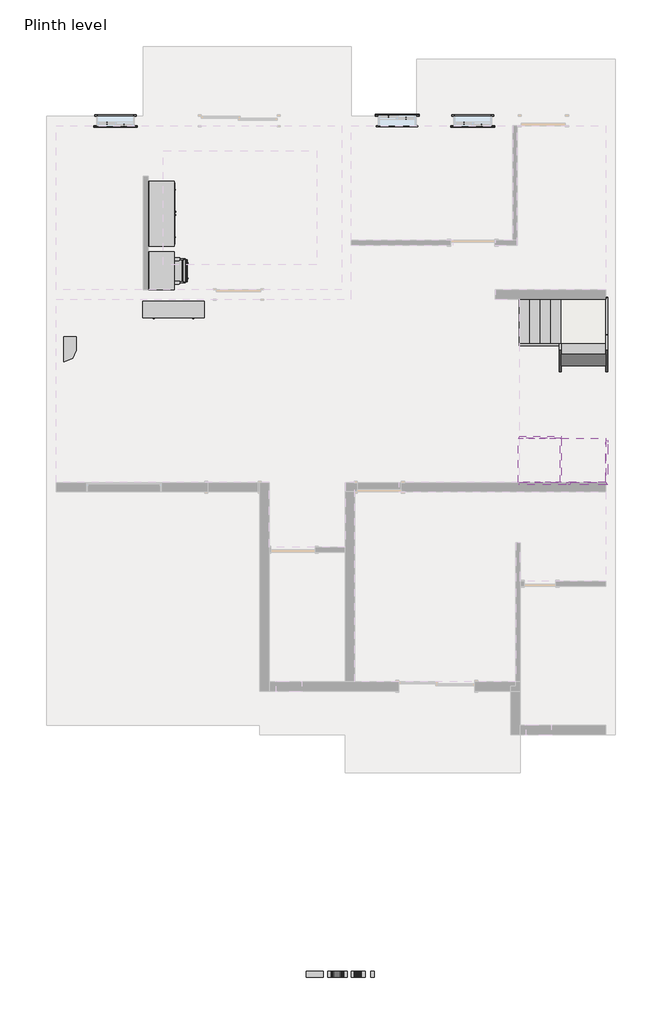
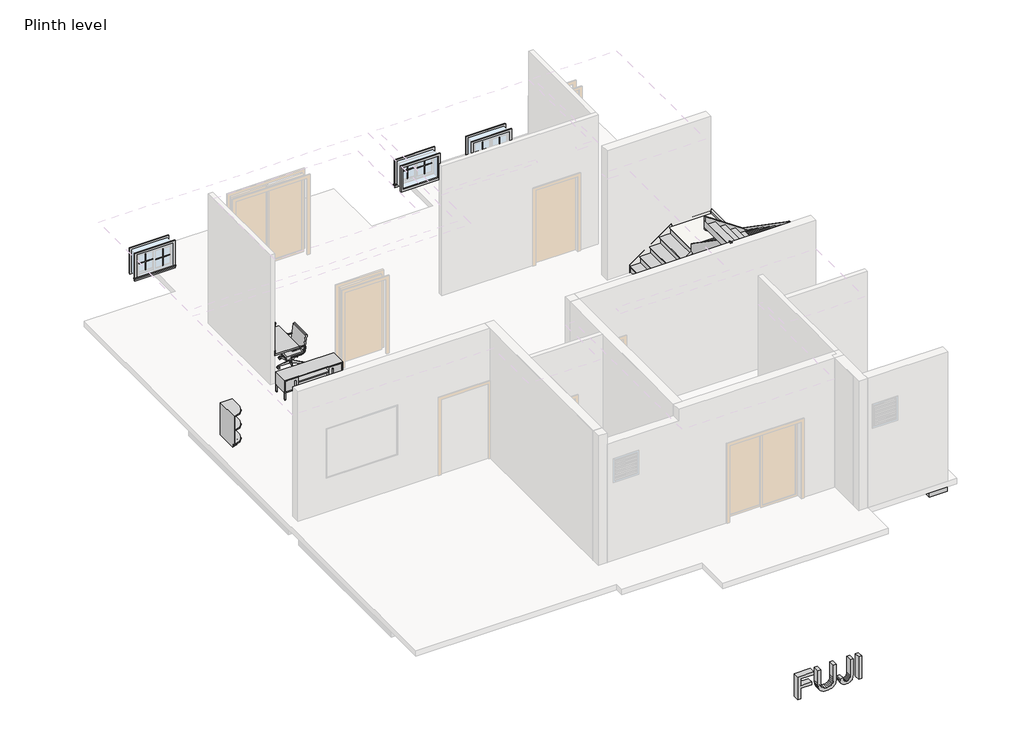
# One storey, part 2 of 2: 25 proxies, 10 members, 7 beams, 6 furniture elements, 3 stair flights, 2 slabs.
"""IFC4 building model written with IfcOpenShell, lengths in millimetres."""

from ifc_helpers import new_model, si_unit, frame, origin, place, context, project, spatial, polyline, outline, extrude, faceted_brep, transform, mapped, element, save
from components import muntin_pattern_2x2_muntin_pattern_2x2_87da473c, trim_window_exterior_flat_with_sill_40e754a6, trim_window_interior_flat_picture_frame_6592d821, furniture_d2b2b685, furniture_4ce329b2, chair_task_arms_chair_task_arms_bb362225, tv_stand_17254_tv_stand_17254_2bb553a4, furniture_0c89dcb9, furniture_49332987, non_monolithic_landing_caa31a54, non_monolithic_landing_665b62c1, stair_flight_49469ed7, stair_flight_6a237a90, stair_flight_f733f96e

model = new_model("IFC4")

# Units and contexts
model_context = context("Model", 3, world=origin())
ifc_project = project(units=[si_unit("LENGTHUNIT", "METRE", prefix="MILLI")], contexts=[model_context])

# Site, building, storey
site = spatial("IfcSite", under=ifc_project)
building = spatial("IfcBuilding", under=site)
storey = spatial("IfcBuildingStorey", under=building, Name="Plinth level", Elevation=0.0)

# Beams
placement = place(None, origin())
element("IfcBeam", 1, ObjectType="Concrete-Rectangular Beam : 18X12", at=placement, inside=storey, context=model_context, shape_type="Brep", body=[
    faceted_brep([(5601.0916032, 10641.5241878, -152.4), (5601.0916032, 10184.3241878, -152.4), (12153.8099466, 10184.3241878, -152.4), (12611.0099466, 10184.3241878, -152.4), (12611.0099466, 10412.9241878, -152.4), (12382.4099466, 10412.9241878, -152.4), (12382.4099466, 10641.5241878, -152.4), (7823.1099466, 10641.5241878, -152.4), (7823.1099466, 10412.9241878, -152.4), (7594.5099466, 10412.9241878, -152.4), (7594.5099466, 10641.5241878, -152.4), (5601.0916032, 10184.3241878, -457.2), (12153.8099466, 10184.3241878, -457.2), (12611.0099466, 10184.3241878, -457.2), (5601.0916032, 10641.5241878, -457.2), (7594.5099466, 10641.5241878, -457.2), (7594.5099466, 10412.9241878, -457.2), (7823.1099466, 10412.9241878, -457.2), (7823.1099466, 10641.5241878, -457.2), (12382.4099466, 10641.5241878, -457.2), (12382.4099466, 10412.9241878, -457.2), (12611.0099466, 10412.9241878, -457.2)], [[[0, 1, 2, 3, 4, 5, 6, 7, 8, 9, 10]], [[1, 11, 12, 13, 3, 2]], [[11, 14, 15, 16, 17, 18, 19, 20, 21, 13, 12]], [[6, 19, 18, 7]], [[0, 14, 11, 1]], [[3, 13, 21, 4]], [[20, 5, 4, 21]], [[5, 20, 19, 6]], [[17, 8, 7, 18]], [[8, 17, 16, 9]], [[9, 16, 15, 10]], [[14, 0, 10, 15]]]),
])
element("IfcBeam", 2, ObjectType="Concrete-Rectangular Beam : 18X12", at=placement, inside=storey, context=model_context, shape_type="Brep", body=[
    faceted_brep([(12611.0099466, 10184.3241878, -152.4), (18402.6916032, 10184.3241878, -152.4), (18859.8916032, 10184.3241878, -152.4), (18859.8916032, 10412.9241878, -152.4), (18402.6916032, 10412.9241878, -152.4), (18402.6916032, 10641.5241878, -152.4), (12839.6099466, 10641.5241878, -152.4), (12839.6099466, 10412.9241878, -152.4), (12611.0099466, 10412.9241878, -152.4), (18859.8916032, 10184.3241878, -457.2), (12611.0099466, 10184.3241878, -457.2), (18402.6916032, 10184.3241878, -457.2), (12611.0099466, 10412.9241878, -457.2), (12839.6099466, 10412.9241878, -457.2), (12839.6099466, 10641.5241878, -457.2), (18402.6916032, 10641.5241878, -457.2), (18402.6916032, 10412.9241878, -457.2), (18859.8916032, 10412.9241878, -457.2)], [[[0, 1, 2, 3, 4, 5, 6, 7, 8]], [[9, 2, 1, 0, 10, 11]], [[9, 11, 10, 12, 13, 14, 15, 16, 17]], [[14, 6, 5, 15]], [[2, 9, 17, 3]], [[10, 0, 8, 12]], [[13, 7, 6, 14]], [[7, 13, 12, 8]], [[16, 4, 3, 17]], [[4, 16, 15, 5]]]),
])
element("IfcBeam", 3, ObjectType="Concrete-Rectangular Beam : 18X12", at=placement, inside=storey, context=model_context, shape_type="Brep", body=[
    faceted_brep([(18859.8916032, 10184.3241878, -152.4), (18402.6916032, 10184.3241878, -152.4), (18402.6916032, 6450.5241878, -152.4), (18823.689508, 6450.5241878, -152.4), (18823.689508, 6221.9241878, -152.4), (18402.6916032, 6221.9241878, -152.4), (18402.6916032, 1802.3241878, -152.4), (18859.8916032, 1802.3241878, -152.4), (18402.6916032, 10184.3241878, -457.2), (18402.6916032, 6450.5241878, -457.2), (18859.8916032, 10184.3241878, -457.2), (18859.8916032, 1802.3241878, -457.2), (18402.6916032, 1802.3241878, -457.2), (18402.6916032, 6221.9241878, -457.2), (18823.689508, 6221.9241878, -457.2), (18823.689508, 6450.5241878, -457.2)], [[[0, 1, 2, 3, 4, 5, 6, 7]], [[1, 8, 9, 2]], [[8, 10, 11, 12, 13, 14, 15, 9]], [[10, 0, 7, 11]], [[1, 0, 10, 8]], [[15, 3, 2, 9]], [[3, 15, 14, 4]], [[4, 14, 13, 5]], [[7, 6, 12, 11]], [[5, 13, 12, 6]]]),
    faceted_brep([(18859.8916032, -4052.3758122, -152.4), (18402.6916032, -4052.3758122, -152.4), (18402.6916032, -4052.3758122, -457.2), (18859.8916032, -4052.3758122, -457.2), (18402.6916032, -3226.8758122, -152.4), (18402.6916032, -2769.6758122, -152.4), (18402.6916032, 1345.1241878, -152.4), (18402.6916032, 1573.7241878, -152.4), (18402.6916032, 1573.7241878, -457.2), (18402.6916032, 1345.1241878, -457.2), (18402.6916032, -2769.6758122, -457.2), (18402.6916032, -3226.8758122, -457.2), (18859.8916032, 1573.7241878, -152.4), (18859.8916032, 1573.7241878, -457.2)], [[[0, 1, 2, 3]], [[2, 1, 4, 5, 6, 7, 8, 9, 10, 11]], [[7, 12, 13, 8]], [[1, 0, 12, 7, 6, 5, 4]], [[3, 2, 11, 10, 9, 8, 13]], [[0, 3, 13, 12]]]),
])
element("IfcBeam", 4, ObjectType="Concrete-Rectangular Beam : 18X12", at=placement, inside=storey, context=model_context, shape_type="Brep", body=[
    faceted_brep([(12611.0099466, 6679.1241878, -152.4), (12153.8099466, 6679.1241878, -152.4), (5829.6916032, 6679.1241878, -152.4), (5829.6916032, 6221.9241878, -152.4), (7480.2099466, 6221.9241878, -152.4), (7480.2099466, 6450.5241878, -152.4), (7708.8099466, 6450.5241878, -152.4), (7708.8099466, 6221.9241878, -152.4), (12153.8099466, 6221.9241878, -152.4), (12153.8099466, 6450.5241878, -152.4), (12611.0099466, 6450.5241878, -152.4), (12153.8099466, 6221.9241878, -457.2), (7708.8099466, 6221.9241878, -457.2), (5829.6916032, 6679.1241878, -457.2), (12153.8099466, 6679.1241878, -457.2), (12611.0099466, 6679.1241878, -457.2), (12611.0099466, 6450.5241878, -457.2), (12153.8099466, 6450.5241878, -457.2), (7708.8099466, 6450.5241878, -457.2), (7480.2099466, 6450.5241878, -457.2), (7480.2099466, 6221.9241878, -457.2), (5829.6916032, 6221.9241878, -457.2)], [[[0, 1, 2, 3, 4, 5, 6, 7, 8, 9, 10]], [[11, 8, 7, 12]], [[13, 14, 15, 16, 17, 11, 12, 18, 19, 20, 21]], [[0, 15, 14, 13, 2, 1]], [[3, 2, 13, 21]], [[15, 0, 10, 16]], [[9, 17, 16, 10]], [[17, 9, 8, 11]], [[6, 18, 12, 7]], [[19, 5, 4, 20]], [[5, 19, 18, 6]], [[3, 21, 20, 4]]]),
])
element("IfcBeam", 5, ObjectType="Concrete-Rectangular Beam : 18X12", at=placement, inside=storey, context=model_context, shape_type="SweptSolid", body=[
    extrude(outline(polyline([(12153.8099466, 10184.3241878), (12611.0099466, 10184.3241878), (12611.0099466, 6679.1241878), (12153.8099466, 6679.1241878), (12153.8099466, 10184.3241878)])), frame((0.0, 0.0, -457.2), z_axis=(0.0, 0.0, 1.0), x_axis=(1.0, 0.0, 0.0)), (0.0, 0.0, 1.0), 304.8),
])
element("IfcBeam", 6, ObjectType="Concrete-Rectangular Beam : 18X12", at=placement, inside=storey, context=model_context, shape_type="Brep", body=[
    faceted_brep([(18402.2099466, 6679.1241878, -152.4), (12611.0099466, 6679.1241878, -152.4), (12611.0099466, 6450.5241878, -152.4), (12611.0099466, 6221.9241878, -152.4), (18366.489508, 6221.9241878, -152.4), (18366.489508, 6450.5241878, -152.4), (18402.2099466, 6450.5241878, -152.4), (12611.0099466, 6221.9241878, -457.2), (18366.489508, 6221.9241878, -457.2), (12611.0099466, 6679.1241878, -457.2), (18402.2099466, 6679.1241878, -457.2), (18402.2099466, 6450.5241878, -457.2), (18366.489508, 6450.5241878, -457.2), (12611.0099466, 6450.5241878, -457.2)], [[[0, 1, 2, 3, 4, 5, 6]], [[3, 7, 8, 4]], [[9, 10, 11, 12, 8, 7, 13]], [[0, 10, 9, 1]], [[3, 2, 1, 9, 13, 7]], [[10, 0, 6, 11]], [[5, 12, 11, 6]], [[12, 5, 4, 8]]]),
])
element("IfcBeam", 7, ObjectType="Concrete-Rectangular Beam : 18X12", at=placement, inside=storey, context=model_context, shape_type="Brep", body=[
    faceted_brep([(12153.8099466, 1802.3241878, -152.4), (12459.0916032, 1802.3241878, -152.4), (12611.0099466, 1802.3241878, -152.4), (12611.0099466, 6221.9241878, -152.4), (12153.8099466, 6221.9241878, -152.4), (12153.8099466, 1802.3241878, -457.2), (12153.8099466, 6221.9241878, -457.2), (12611.0099466, 1802.3241878, -457.2), (12459.0916032, 1802.3241878, -457.2), (12611.0099466, 6221.9241878, -457.2)], [[[0, 1, 2, 3, 4]], [[5, 0, 4, 6]], [[7, 8, 5, 6, 9]], [[9, 3, 2, 7]], [[4, 3, 9, 6]], [[0, 5, 8, 7, 2, 1]]]),
])

# Proxies
element("IfcBuildingElementProxy", 8, Name="24\" Arial", ObjectType="24\" Arial", at=placement, inside=storey, context=model_context, shape_type="SweptSolid", body=[
    extrude(outline(polyline([(166.9415952, 11521.8900369), (166.9415952, 11598.0318104), (442.9555242, 11598.0318104), (442.9555242, 11883.5634611), (519.0972977, 11883.5634611), (519.0972977, 11598.0318104), (699.9340098, 11598.0318104), (699.9340098, 11931.1520695), (776.0757833, 11931.1520695), (776.0757833, 11521.8900369), (166.9415952, 11521.8900369)])), frame((0.0, -10135.6758122, 0.0), z_axis=(0.0, 1.0, 0.0), x_axis=(0.0, 0.0, 1.0)), (0.0, 0.0, 1.0), 152.4),
    extrude(outline(polyline([(776.0757833, 12435.5913191), (427.340512, 12435.5913191), (375.0673999, 12433.1840047), (332.0145807, 12425.9620616), (298.1820544, 12413.9254897), (273.569821, 12397.0742891), (256.0679949, 12374.5719413), (243.5666905, 12345.5819276), (236.0659079, 12310.1042483), (233.565647, 12268.1389031), (238.6219367, 12219.2862223), (253.7908056, 12178.6128335), (264.9676223, 12161.6686864), (278.2729139, 12147.4199878), (293.7066804, 12135.8667377), (311.2689217, 12127.0089362), (358.9132981, 12115.7438203), (427.340512, 12111.9887816), (776.0757833, 12111.9887816), (776.0757833, 12035.8470081), (424.6636528, 12035.8470081), (378.8828538, 12037.2923262), (338.2048177, 12041.6282805), (302.6295445, 12048.8548709), (272.1570342, 12058.9720975), (245.8857057, 12072.4679295), (222.913978, 12089.8303358), (203.2418511, 12111.0593166), (186.869325, 12136.1548719), (173.9869399, 12165.1216489), (164.7852364, 12197.964295), (159.2642142, 12234.6828101), (157.4238735, 12275.2771944), (159.5384064, 12316.8986375), (165.8820051, 12354.3188987), (176.4546695, 12387.5379781), (191.2563998, 12416.5558757), (209.4274407, 12441.4004754), (230.1080372, 12462.0996611), (253.2981891, 12478.6534329), (278.9978966, 12491.0617908), (308.3178703, 12500.1054853), (342.3688209, 12506.5652672), (424.6636528, 12511.7330926), (776.0757833, 12511.7330926), (776.0757833, 12435.5913191)])), frame((0.0, -10135.6758122, 0.0), z_axis=(0.0, 1.0, 0.0), x_axis=(0.0, 0.0, 1.0)), (0.0, 0.0, 1.0), 152.4),
    extrude(outline(polyline([(337.9631568, 12606.9103095), (295.8909232, 12608.8435967), (259.3490063, 12616.2793168), (228.3374063, 12629.2174697), (202.8561231, 12647.6580555), (182.9795139, 12671.1828149), (168.7819359, 12699.3734886), (160.2633891, 12732.2300766), (157.4238735, 12769.752579), (162.9263063, 12819.9994574), (169.8043474, 12842.5436312), (179.4336049, 12863.3682947), (191.6793064, 12881.9854788), (206.4066794, 12897.9072144), (223.6157241, 12911.1335015), (243.3064403, 12921.6643401), (266.3989984, 12929.6995651), (293.8135689, 12935.4390115), (361.6087466, 12940.0305686), (776.0757833, 12940.0305686), (776.0757833, 12863.8887951), (360.270317, 12863.8887951), (315.5258715, 12861.8253828), (284.7977583, 12855.6351458), (263.5687775, 12843.9610653), (247.3217291, 12825.4461224), (237.0046675, 12801.4473358), (233.565647, 12773.3217247), (235.080675, 12753.9144953), (239.6257589, 12736.7379819), (247.2008987, 12721.7921846), (257.8060944, 12709.0771033), (272.5195255, 12698.750747), (292.4193714, 12690.9711249), (317.5056319, 12685.7382369), (347.7783073, 12683.052083), (337.9631568, 12606.9103095)])), frame((0.0, -10135.6758122, 0.0), z_axis=(0.0, 1.0, 0.0), x_axis=(0.0, 0.0, 1.0)), (0.0, 0.0, 1.0), 152.4),
    extrude(outline(polyline([(13158.9381675, -10135.6758122), (13082.796394, -10135.6758122), (13082.796394, -9983.2758122), (13158.9381675, -9983.2758122), (13158.9381675, -10135.6758122)])), frame((0.0, 0.0, 166.9415952), z_axis=(0.0, 0.0, 1.0), x_axis=(1.0, 0.0, 0.0)), (0.0, 0.0, 1.0), 609.1341881),
])
muntin_pattern_2x2_muntin_pattern_2x2_shape = muntin_pattern_2x2_muntin_pattern_2x2_87da473c(model_context)
element("IfcBuildingElementProxy", 9, Name="Muntin Pattern_2x2 : Muntin Pattern_2x2", ObjectType="Muntin Pattern_2x2 : Muntin Pattern_2x2", at=placement, inside=storey, context=model_context, shape_type="MappedRepresentation", body=[
    mapped(muntin_pattern_2x2_muntin_pattern_2x2_shape, transform((6713.9291032, 10466.8991878, 996.95), x_axis=(-1.0, 0.0, 0.0), y_axis=(0.0, -1.0, 0.0), z_axis=(0.0, 0.0, 1.0))),
])
element("IfcBuildingElementProxy", 10, Name="Muntin Pattern_2x2 : Muntin Pattern_2x2", ObjectType="Muntin Pattern_2x2 : Muntin Pattern_2x2", at=placement, inside=storey, context=model_context, shape_type="MappedRepresentation", body=[
    mapped(muntin_pattern_2x2_muntin_pattern_2x2_shape, transform((7129.8541032, 10422.4491878, 996.95), x_axis=(-1.0, 0.0, 0.0), y_axis=(0.0, -1.0, 0.0), z_axis=(0.0, 0.0, 1.0))),
])
element("IfcBuildingElementProxy", 11, Name="Muntin Pattern_2x2 : Muntin Pattern_2x2", ObjectType="Muntin Pattern_2x2 : Muntin Pattern_2x2", at=placement, inside=storey, context=model_context, shape_type="MappedRepresentation", body=[
    mapped(muntin_pattern_2x2_muntin_pattern_2x2_shape, transform((13923.8724466, 10587.5491878, 996.95), x_axis=(1.0, 0.0, 0.0), y_axis=(0.0, 1.0, 0.0), z_axis=(0.0, 0.0, 1.0))),
])
element("IfcBuildingElementProxy", 12, Name="Muntin Pattern_2x2 : Muntin Pattern_2x2", ObjectType="Muntin Pattern_2x2 : Muntin Pattern_2x2", at=placement, inside=storey, context=model_context, shape_type="MappedRepresentation", body=[
    mapped(muntin_pattern_2x2_muntin_pattern_2x2_shape, transform((13507.9474466, 10631.9991878, 996.95), x_axis=(1.0, 0.0, 0.0), y_axis=(0.0, 1.0, 0.0), z_axis=(0.0, 0.0, 1.0))),
])
element("IfcBuildingElementProxy", 13, Name="Muntin Pattern_2x2 : Muntin Pattern_2x2", ObjectType="Muntin Pattern_2x2 : Muntin Pattern_2x2", at=placement, inside=storey, context=model_context, shape_type="MappedRepresentation", body=[
    mapped(muntin_pattern_2x2_muntin_pattern_2x2_shape, transform((15330.3974466, 10466.8991878, 996.95), x_axis=(-1.0, 0.0, 0.0), y_axis=(0.0, -1.0, 0.0), z_axis=(0.0, 0.0, 1.0))),
])
element("IfcBuildingElementProxy", 14, Name="Muntin Pattern_2x2 : Muntin Pattern_2x2", ObjectType="Muntin Pattern_2x2 : Muntin Pattern_2x2", at=placement, inside=storey, context=model_context, shape_type="MappedRepresentation", body=[
    mapped(muntin_pattern_2x2_muntin_pattern_2x2_shape, transform((15746.3224466, 10422.4491878, 996.95), x_axis=(-1.0, 0.0, 0.0), y_axis=(0.0, -1.0, 0.0), z_axis=(0.0, 0.0, 1.0))),
])
element("IfcBuildingElementProxy", 15, Name="Muntin Pattern_2x2 : Muntin Pattern_2x2", ObjectType="Muntin Pattern_2x2 : Muntin Pattern_2x2", at=placement, inside=storey, context=model_context, shape_type="MappedRepresentation", body=[
    mapped(muntin_pattern_2x2_muntin_pattern_2x2_shape, transform((6713.9291032, 10466.8991878, 996.95), x_axis=(-1.0, 0.0, 0.0), y_axis=(0.0, -1.0, 0.0), z_axis=(0.0, 0.0, 1.0))),
])
element("IfcBuildingElementProxy", 16, Name="Muntin Pattern_2x2 : Muntin Pattern_2x2", ObjectType="Muntin Pattern_2x2 : Muntin Pattern_2x2", at=placement, inside=storey, context=model_context, shape_type="MappedRepresentation", body=[
    mapped(muntin_pattern_2x2_muntin_pattern_2x2_shape, transform((7129.8541032, 10422.4491878, 996.95), x_axis=(-1.0, 0.0, 0.0), y_axis=(0.0, -1.0, 0.0), z_axis=(0.0, 0.0, 1.0))),
])
element("IfcBuildingElementProxy", 17, Name="Muntin Pattern_2x2 : Muntin Pattern_2x2", ObjectType="Muntin Pattern_2x2 : Muntin Pattern_2x2", at=placement, inside=storey, context=model_context, shape_type="MappedRepresentation", body=[
    mapped(muntin_pattern_2x2_muntin_pattern_2x2_shape, transform((13923.8724466, 10587.5491878, 996.95), x_axis=(1.0, 0.0, 0.0), y_axis=(0.0, 1.0, 0.0), z_axis=(0.0, 0.0, 1.0))),
])
element("IfcBuildingElementProxy", 18, Name="Muntin Pattern_2x2 : Muntin Pattern_2x2", ObjectType="Muntin Pattern_2x2 : Muntin Pattern_2x2", at=placement, inside=storey, context=model_context, shape_type="MappedRepresentation", body=[
    mapped(muntin_pattern_2x2_muntin_pattern_2x2_shape, transform((13507.9474466, 10631.9991878, 996.95), x_axis=(1.0, 0.0, 0.0), y_axis=(0.0, 1.0, 0.0), z_axis=(0.0, 0.0, 1.0))),
])
element("IfcBuildingElementProxy", 19, Name="Muntin Pattern_2x2 : Muntin Pattern_2x2", ObjectType="Muntin Pattern_2x2 : Muntin Pattern_2x2", at=placement, inside=storey, context=model_context, shape_type="MappedRepresentation", body=[
    mapped(muntin_pattern_2x2_muntin_pattern_2x2_shape, transform((15330.3974466, 10466.8991878, 996.95), x_axis=(-1.0, 0.0, 0.0), y_axis=(0.0, -1.0, 0.0), z_axis=(0.0, 0.0, 1.0))),
])
element("IfcBuildingElementProxy", 20, Name="Muntin Pattern_2x2 : Muntin Pattern_2x2", ObjectType="Muntin Pattern_2x2 : Muntin Pattern_2x2", at=placement, inside=storey, context=model_context, shape_type="MappedRepresentation", body=[
    mapped(muntin_pattern_2x2_muntin_pattern_2x2_shape, transform((15746.3224466, 10422.4491878, 996.95), x_axis=(-1.0, 0.0, 0.0), y_axis=(0.0, -1.0, 0.0), z_axis=(0.0, 0.0, 1.0))),
])
trim_window_exterior_flat_with_sill_shape = trim_window_exterior_flat_with_sill_40e754a6(model_context)
element("IfcBuildingElementProxy", 21, Name="Trim-Window-Exterior-Flat : with Sill", ObjectType="Trim-Window-Exterior-Flat : with Sill", at=placement, inside=storey, context=model_context, shape_type="MappedRepresentation", body=[
    mapped(trim_window_exterior_flat_with_sill_shape, transform((6921.8916032, 10412.9241878, 1524.0), x_axis=(1.0, 0.0, 0.0), y_axis=(0.0, 0.0, 1.0), z_axis=(0.0, -1.0, 0.0))),
])
element("IfcBuildingElementProxy", 22, Name="Trim-Window-Exterior-Flat : with Sill", ObjectType="Trim-Window-Exterior-Flat : with Sill", at=placement, inside=storey, context=model_context, shape_type="MappedRepresentation", body=[
    mapped(trim_window_exterior_flat_with_sill_shape, transform((13715.9099466, 10641.5241878, 1524.0), x_axis=(-1.0, 0.0, 0.0), y_axis=(0.0, 0.0, 1.0), z_axis=(0.0, 1.0, 0.0))),
])
element("IfcBuildingElementProxy", 23, Name="Trim-Window-Exterior-Flat : with Sill", ObjectType="Trim-Window-Exterior-Flat : with Sill", at=placement, inside=storey, context=model_context, shape_type="MappedRepresentation", body=[
    mapped(trim_window_exterior_flat_with_sill_shape, transform((15538.3599466, 10412.9241878, 1524.0), x_axis=(1.0, 0.0, 0.0), y_axis=(0.0, 0.0, 1.0), z_axis=(0.0, -1.0, 0.0))),
])
element("IfcBuildingElementProxy", 24, Name="Trim-Window-Exterior-Flat : with Sill", ObjectType="Trim-Window-Exterior-Flat : with Sill", at=placement, inside=storey, context=model_context, shape_type="MappedRepresentation", body=[
    mapped(trim_window_exterior_flat_with_sill_shape, transform((6921.8916032, 10412.9241878, 1524.0), x_axis=(1.0, 0.0, 0.0), y_axis=(0.0, 0.0, 1.0), z_axis=(0.0, -1.0, 0.0))),
])
element("IfcBuildingElementProxy", 25, Name="Trim-Window-Exterior-Flat : with Sill", ObjectType="Trim-Window-Exterior-Flat : with Sill", at=placement, inside=storey, context=model_context, shape_type="MappedRepresentation", body=[
    mapped(trim_window_exterior_flat_with_sill_shape, transform((13715.9099466, 10641.5241878, 1524.0), x_axis=(-1.0, 0.0, 0.0), y_axis=(0.0, 0.0, 1.0), z_axis=(0.0, 1.0, 0.0))),
])
element("IfcBuildingElementProxy", 26, Name="Trim-Window-Exterior-Flat : with Sill", ObjectType="Trim-Window-Exterior-Flat : with Sill", at=placement, inside=storey, context=model_context, shape_type="MappedRepresentation", body=[
    mapped(trim_window_exterior_flat_with_sill_shape, transform((15538.3599466, 10412.9241878, 1524.0), x_axis=(1.0, 0.0, 0.0), y_axis=(0.0, 0.0, 1.0), z_axis=(0.0, -1.0, 0.0))),
])
trim_window_interior_flat_picture_frame_shape = trim_window_interior_flat_picture_frame_6592d821(model_context)
element("IfcBuildingElementProxy", 27, Name="Trim-Window-Interior-Flat : Picture Frame", ObjectType="Trim-Window-Interior-Flat : Picture Frame", at=placement, inside=storey, context=model_context, shape_type="MappedRepresentation", body=[
    mapped(trim_window_interior_flat_picture_frame_shape, transform((6921.8916032, 10641.5241878, 1524.0), x_axis=(-1.0, 0.0, 0.0), y_axis=(0.0, 0.0, 1.0), z_axis=(0.0, 1.0, 0.0))),
])
element("IfcBuildingElementProxy", 28, Name="Trim-Window-Interior-Flat : Picture Frame", ObjectType="Trim-Window-Interior-Flat : Picture Frame", at=placement, inside=storey, context=model_context, shape_type="MappedRepresentation", body=[
    mapped(trim_window_interior_flat_picture_frame_shape, transform((13715.9099466, 10412.9241878, 1524.0), x_axis=(1.0, 0.0, 0.0), y_axis=(0.0, 0.0, 1.0), z_axis=(0.0, -1.0, 0.0))),
])
element("IfcBuildingElementProxy", 29, Name="Trim-Window-Interior-Flat : Picture Frame", ObjectType="Trim-Window-Interior-Flat : Picture Frame", at=placement, inside=storey, context=model_context, shape_type="MappedRepresentation", body=[
    mapped(trim_window_interior_flat_picture_frame_shape, transform((15538.3599466, 10641.5241878, 1524.0), x_axis=(-1.0, 0.0, 0.0), y_axis=(0.0, 0.0, 1.0), z_axis=(0.0, 1.0, 0.0))),
])
element("IfcBuildingElementProxy", 30, Name="Trim-Window-Interior-Flat : Picture Frame", ObjectType="Trim-Window-Interior-Flat : Picture Frame", at=placement, inside=storey, context=model_context, shape_type="MappedRepresentation", body=[
    mapped(trim_window_interior_flat_picture_frame_shape, transform((6921.8916032, 10641.5241878, 1524.0), x_axis=(-1.0, 0.0, 0.0), y_axis=(0.0, 0.0, 1.0), z_axis=(0.0, 1.0, 0.0))),
])
element("IfcBuildingElementProxy", 31, Name="Trim-Window-Interior-Flat : Picture Frame", ObjectType="Trim-Window-Interior-Flat : Picture Frame", at=placement, inside=storey, context=model_context, shape_type="MappedRepresentation", body=[
    mapped(trim_window_interior_flat_picture_frame_shape, transform((13715.9099466, 10412.9241878, 1524.0), x_axis=(1.0, 0.0, 0.0), y_axis=(0.0, 0.0, 1.0), z_axis=(0.0, -1.0, 0.0))),
])
element("IfcBuildingElementProxy", 32, Name="Trim-Window-Interior-Flat : Picture Frame", ObjectType="Trim-Window-Interior-Flat : Picture Frame", at=placement, inside=storey, context=model_context, shape_type="MappedRepresentation", body=[
    mapped(trim_window_interior_flat_picture_frame_shape, transform((15538.3599466, 10641.5241878, 1524.0), x_axis=(-1.0, 0.0, 0.0), y_axis=(0.0, 0.0, 1.0), z_axis=(0.0, 1.0, 0.0))),
])

# Furniture
furniture_shape = furniture_d2b2b685(model_context)
element("IfcFurniture", 33, ObjectType="48\"", at=placement, inside=storey, context=model_context, shape_type="MappedRepresentation", body=[
    mapped(furniture_shape, transform((7734.2099466, 8201.1792278, 0.0), x_axis=(0.0, 1.0, 0.0), y_axis=(-1.0, 0.0, 0.0), z_axis=(0.0, 0.0, 1.0))),
])
furniture_2_shape = furniture_4ce329b2(model_context)
element("IfcFurniture", 34, ObjectType="Base Cabinet-End w Shelves : 12\"", at=placement, inside=storey, context=model_context, shape_type="MappedRepresentation", body=[
    mapped(furniture_2_shape, transform((5670.4599466, 5320.2241878, 0.0), x_axis=(1.0, 0.0, 0.0), y_axis=(0.0, 1.0, 0.0), z_axis=(0.0, 0.0, 1.0))),
])
chair_task_arms_chair_task_arms_shape = chair_task_arms_chair_task_arms_bb362225(model_context)
element("IfcFurniture", 35, ObjectType="Chair-Task Arms : Chair-Task Arms", at=placement, inside=storey, context=model_context, shape_type="MappedRepresentation", body=[
    mapped(chair_task_arms_chair_task_arms_shape, transform((8401.3375049, 6766.7333681, 0.0), x_axis=(0.0, 1.0, 0.0), y_axis=(-1.0, 0.0, 0.0), z_axis=(0.0, 0.0, 1.0))),
])
tv_stand_17254_tv_stand_17254_shape = tv_stand_17254_tv_stand_17254_2bb553a4(model_context)
element("IfcFurniture", 36, ObjectType="TV_Stand_17254 : TV_Stand_17254", at=placement, inside=storey, context=model_context, shape_type="MappedRepresentation", body=[
    mapped(tv_stand_17254_tv_stand_17254_shape, transform((8318.4099466, 6171.1241878, 0.0), x_axis=(-1.0, 0.0, 0.0), y_axis=(0.0, -1.0, 0.0), z_axis=(0.0, 0.0, 1.0))),
])
furniture_3_shape = furniture_0c89dcb9(model_context)
element("IfcFurniture", 37, ObjectType="Vanity Counter Top : 24\" Depth", at=placement, inside=storey, context=model_context, shape_type="MappedRepresentation", body=[
    mapped(furniture_3_shape, transform((7708.8099466, 7650.9864829, 0.0), x_axis=(0.0, 1.0, 0.0), y_axis=(-1.0, 0.0, 0.0), z_axis=(0.0, 0.0, 1.0))),
])
furniture_4_shape = furniture_49332987(model_context)
element("IfcFurniture", 38, ObjectType="Vanity Counter Top : 24\" Depth", at=placement, inside=storey, context=model_context, shape_type="MappedRepresentation", body=[
    mapped(furniture_4_shape, transform((7708.8099466, 8697.580465, 0.0), x_axis=(0.0, 1.0, 0.0), y_axis=(-1.0, 0.0, 0.0), z_axis=(0.0, 0.0, 1.0))),
])

# Members
element("IfcMember", 39, ObjectType="Stringer - 2\" Width", at=placement, inside=storey, context=model_context, shape_type="SweptSolid", body=[
    extrude(outline(polyline([(220.4595872, 16662.7916032), (0.0, 16662.7916032), (0.0, 16879.9752749), (647.7, 17818.6709271), (952.5, 17723.7197377), (220.4595872, 16662.7916032)])), frame((0.0, 6221.9241878, 0.0), z_axis=(0.0, 1.0, 0.0), x_axis=(0.0, 0.0, 1.0)), (0.0, 0.0, 1.0), 50.8),
])
element("IfcMember", 40, ObjectType="Stringer - 2\" Width", at=placement, inside=storey, context=model_context, shape_type="Brep", body=[
    faceted_brep([(16662.7916032, 5104.3241878, 0.0), (16662.7916032, 5155.1241878, 0.0), (16879.9752749, 5155.1241878, 0.0), (16879.9752749, 5104.3241878, 0.0), (16662.7916032, 5104.3241878, 220.4595872), (16662.7916032, 5155.1241878, 220.4595872), (17627.9916032, 5104.3241878, 886.4475872), (17627.9916032, 5155.1241878, 886.4475872), (17627.9916032, 5155.1241878, 726.4432665), (17627.9916032, 5155.1241878, 516.1312665), (17627.9916032, 5104.3241878, 516.1312665)], [[[0, 1, 2, 3]], [[4, 5, 1, 0]], [[5, 4, 6, 7]], [[1, 5, 7, 8, 9, 2]], [[4, 0, 3, 10, 6]], [[2, 9, 10, 3]], [[6, 10, 9, 8, 7]]]),
])
element("IfcMember", 41, ObjectType="Stringer - 2\" Width", at=placement, inside=storey, context=model_context, shape_type="SweptSolid", body=[
    extrude(outline(polyline([(5364.1960533, 952.5), (5269.2448639, 647.7), (2729.2448639, 2400.3), (2824.1960533, 2705.1), (5364.1960533, 952.5)])), frame((18745.5916032, 0.0, 0.0), z_axis=(1.0, 0.0, 0.0), x_axis=(0.0, 1.0, 0.0)), (0.0, 0.0, 1.0), 50.8),
])
element("IfcMember", 42, ObjectType="Stringer - 2\" Width", at=placement, inside=storey, context=model_context, shape_type="Brep", body=[
    faceted_brep([(17678.7916032, 5155.1241878, 1096.7595872), (17627.9916032, 5155.1241878, 1096.7595872), (17627.9916032, 2919.9241878, 2639.0475872), (17678.7916032, 2919.9241878, 2639.0475872), (17678.7916032, 5155.1241878, 726.4432665), (17678.7916032, 2919.9241878, 2479.0432665), (17678.7916032, 2919.9241878, 2268.7312665), (17627.9916032, 5155.1241878, 726.4432665), (17627.9916032, 2919.9241878, 2268.7312665), (17627.9916032, 5155.1241878, 886.4475872)], [[[0, 1, 2, 3]], [[4, 0, 3, 5, 6]], [[7, 4, 6, 8]], [[1, 9, 7, 8, 2]], [[1, 0, 4, 7, 9]], [[2, 8, 6, 5, 3]]]),
])
element("IfcMember", 43, ObjectType="Stringer - 2\" Width", at=placement, inside=storey, context=model_context, shape_type="Brep", body=[
    faceted_brep([(18745.5916032, 5364.1960533, 952.5), (18796.3916032, 5364.1960533, 952.5), (18796.3916032, 6272.7241878, 952.5), (18745.5916032, 6221.9241878, 952.5), (18745.5916032, 5269.2448639, 647.7), (18745.5916032, 6221.9241878, 647.7), (18796.3916032, 5269.2448639, 647.7), (18796.3916032, 6272.7241878, 647.7)], [[[0, 1, 2, 3]], [[4, 0, 3, 5]], [[6, 4, 5, 7]], [[1, 6, 7, 2]], [[1, 0, 4, 6]], [[2, 7, 5, 3]]]),
])
element("IfcMember", 44, ObjectType="Stringer - 2\" Width", at=placement, inside=storey, context=model_context, shape_type="Brep", body=[
    faceted_brep([(18745.5916032, 6221.9241878, 952.5), (18796.3916032, 6272.7241878, 952.5), (17723.7197377, 6272.7241878, 952.5), (17723.7197377, 6221.9241878, 952.5), (18745.5916032, 6221.9241878, 647.7), (17818.6709271, 6221.9241878, 647.7), (18796.3916032, 6272.7241878, 647.7), (17818.6709271, 6272.7241878, 647.7)], [[[0, 1, 2, 3]], [[4, 0, 3, 5]], [[6, 4, 5, 7]], [[1, 6, 7, 2]], [[1, 0, 4, 6]], [[2, 7, 5, 3]]]),
])
element("IfcMember", 45, ObjectType="Stringer - 2\" Width", at=placement, inside=storey, context=model_context, shape_type="SweptSolid", body=[
    extrude(outline(polyline([(2400.3, 17792.9122794), (2705.1, 17887.8634687), (3550.3995872, 16662.7916032), (3180.0832665, 16662.7916032), (2400.3, 17792.9122794)])), frame((0.0, 1751.5241878, 0.0), z_axis=(0.0, 1.0, 0.0), x_axis=(0.0, 0.0, 1.0)), (0.0, 0.0, 1.0), 50.8),
])
element("IfcMember", 46, ObjectType="Stringer - 2\" Width", at=placement, inside=storey, context=model_context, shape_type="Brep", body=[
    faceted_brep([(16662.7916032, 2919.9241878, 3550.3995872), (16662.7916032, 2919.9241878, 3180.0832665), (16662.7916032, 2869.1241878, 3180.0832665), (16662.7916032, 2869.1241878, 3550.3995872), (17678.7916032, 2869.1241878, 2849.3595872), (17678.7916032, 2919.9241878, 2849.3595872), (17678.7916032, 2869.1241878, 2479.0432665), (17678.7916032, 2919.9241878, 2479.0432665), (17678.7916032, 2919.9241878, 2639.0475872)], [[[0, 1, 2, 3]], [[4, 5, 0, 3]], [[6, 4, 3, 2]], [[7, 6, 2, 1]], [[5, 8, 7, 1, 0]], [[5, 4, 6, 7, 8]]]),
])
element("IfcMember", 47, ObjectType="Stringer - 2\" Width", at=placement, inside=storey, context=model_context, shape_type="Brep", body=[
    faceted_brep([(17887.8634687, 1802.3241878, 2705.1), (17887.8634687, 1751.5241878, 2705.1), (18796.3916032, 1751.5241878, 2705.1), (18745.5916032, 1802.3241878, 2705.1), (17792.9122794, 1802.3241878, 2400.3), (18745.5916032, 1802.3241878, 2400.3), (17792.9122794, 1751.5241878, 2400.3), (18796.3916032, 1751.5241878, 2400.3)], [[[0, 1, 2, 3]], [[4, 0, 3, 5]], [[6, 4, 5, 7]], [[1, 6, 7, 2]], [[1, 0, 4, 6]], [[2, 7, 5, 3]]]),
])
element("IfcMember", 48, ObjectType="Stringer - 2\" Width", at=placement, inside=storey, context=model_context, shape_type="Brep", body=[
    faceted_brep([(18745.5916032, 1802.3241878, 2705.1), (18796.3916032, 1751.5241878, 2705.1), (18796.3916032, 2824.1960533, 2705.1), (18745.5916032, 2824.1960533, 2705.1), (18745.5916032, 1802.3241878, 2400.3), (18745.5916032, 2729.2448639, 2400.3), (18796.3916032, 1751.5241878, 2400.3), (18796.3916032, 2729.2448639, 2400.3)], [[[0, 1, 2, 3]], [[4, 0, 3, 5]], [[6, 4, 5, 7]], [[1, 6, 7, 2]], [[1, 0, 4, 6]], [[2, 7, 5, 3]]]),
])

# Slabs
non_monolithic_landing_shape = non_monolithic_landing_caa31a54(model_context)
element("IfcSlab", 49, ObjectType="Non-Monolithic Landing", at=placement, inside=storey, context=model_context, shape_type="MappedRepresentation", body=[
    mapped(non_monolithic_landing_shape, transform((0.0, 0.0, 0.0), x_axis=(1.0, 0.0, 0.0), y_axis=(0.0, 1.0, 0.0), z_axis=(0.0, 0.0, 1.0))),
])
non_monolithic_landing_2_shape = non_monolithic_landing_665b62c1(model_context)
element("IfcSlab", 50, ObjectType="Non-Monolithic Landing", at=placement, inside=storey, context=model_context, shape_type="MappedRepresentation", body=[
    mapped(non_monolithic_landing_2_shape, transform((0.0, 0.0, 0.0), x_axis=(1.0, 0.0, 0.0), y_axis=(0.0, 1.0, 0.0), z_axis=(0.0, 0.0, 1.0))),
])

# Stair flights
stair_flight_shape = stair_flight_49469ed7(model_context)
element("IfcStairFlight", 51, ObjectType="2\" Tread 1\" Nosing 1/4\" Riser", at=placement, inside=storey, context=model_context, shape_type="MappedRepresentation", body=[
    mapped(stair_flight_shape, transform((0.0, 0.0, 0.0), x_axis=(1.0, 0.0, 0.0), y_axis=(0.0, 1.0, 0.0), z_axis=(0.0, 0.0, 1.0))),
])
stair_flight_2_shape = stair_flight_6a237a90(model_context)
element("IfcStairFlight", 52, ObjectType="2\" Tread 1\" Nosing 1/4\" Riser", at=placement, inside=storey, context=model_context, shape_type="MappedRepresentation", body=[
    mapped(stair_flight_2_shape, transform((0.0, 0.0, 0.0), x_axis=(1.0, 0.0, 0.0), y_axis=(0.0, 1.0, 0.0), z_axis=(0.0, 0.0, 1.0))),
])
stair_flight_3_shape = stair_flight_f733f96e(model_context)
element("IfcStairFlight", 53, ObjectType="2\" Tread 1\" Nosing 1/4\" Riser", at=placement, inside=storey, context=model_context, shape_type="MappedRepresentation", body=[
    mapped(stair_flight_3_shape, transform((0.0, 0.0, 0.0), x_axis=(1.0, 0.0, 0.0), y_axis=(0.0, 1.0, 0.0), z_axis=(0.0, 0.0, 1.0))),
])

save(model, "model.ifc")

# Revit data of these elements
# Type "Concrete-Rectangular Beam : 18X12"
#   Assembly Code = "B10"
#   Length [instance default] = 5' - 0"
#   b = 1' - 6"
#   h = 1' - 0"
#   Structural Material [instance default] = Concrete, Cast-in-Place gray
# Type "Muntin Pattern_2x2 : Muntin Pattern_2x2"
#   Width [instance default] = 4' - 0"
#   Thickness = 0' - 0 1/2"
#   Height [instance default] = 4' - 0"
#   Distance = 0' - 0 3/4"
#   Interior Material [instance default] = none
#   Exterior Material [instance default] = none
#   Default Elevation = 0
# Type "Trim-Window-Exterior-Flat : with Sill"
#   Trim Width = 0' - 2 1/4"
#   Trim Thickness_Picture Frame = 0' - 1 1/4"
#   Trim Thickness_with Sill = 0' - 0 3/4"
#   Sill Thickness = 0' - 1 1/4"
#   Opening Width [instance default] = 2' - 0"
#   Opening Height [instance default] = 3' - 0"
#   Default Elevation = 4' - 0"
#   Sill = yes
#   Picture Frame = no
#   Trim Material [instance default] = none
# Type "Trim-Window-Interior-Flat : Picture Frame"
#   Trim Thickness_Picture Frame = 0' - 1 1/4"
#   Trim Width = 0' - 2 1/4"
#   Trim Thickness_with Sill = 0' - 0 3/4"
#   Sill Thickness = 0' - 1 1/4"
#   Opening Width [instance default] = 2' - 0"
#   Opening Height [instance default] = 3' - 0"
#   Default Elevation = 4' - 0"
#   Sill = no
#   Picture Frame = yes
#   Trim Material [instance default] = none
# Type "48\""
#   Assembly Code = "C1030410"
#   Depth = 2' - 0"
#   Height = 2' - 5 1/2"
#   Toe Depth = 0' - 3"
#   Toe Height = 0' - 3 1/2"
#   Width = 5' - 0"
#   Cabinet Material = none
#   Door/Drawer Material = none
#   Handle Material = Cabinets - Handles
#   Default Elevation = 0
# Type "Base Cabinet-End w Shelves : 12\""
#   Assembly Code = "C1030410"
#   Width = 1' - 0"
#   Toe Kick Depth = 0' - 3"
#   Height = 2' - 10 1/2"
#   Depth = 2' - 0"
#   Cabinet Material = Cabinets
#   Default Elevation = 0
# Type "Chair-Task Arms : Chair-Task Arms"
#   Assembly Code = "E2020200"
#   Base Material = Plastic, Opaque Black
#   Caster Material = Plastic, Opaque Black
#   Seat/Back Material = Textile - Slate Blue
#   Default Elevation = 0
# Type "TV_Stand_17254 : TV_Stand_17254"
#   URL = "http://www.woodwaves.com/products/modern-tv-stand-terra-mar-clove"
#   Stand Width = 4' - 10.26772"
#   Stand Height = 1' - 8.86614"
#   Cupboard Width = 1' - 1.38583"
#   Modern TV Stand - White Wood = Modern TV Stand - White Wood
#   Modern TV Stand - Semi Polished = Modern TV Stand - Semi Polished
#   Modern TV Stand - Oak Wood = Modern TV Stand - Oak Wood
#   Default Elevation = 0
# Type "Vanity Counter Top : 24\" Depth"
#   Counter Thickness = 0' - 1 1/2"
#   Depth = 2' - 1"
#   Height = 2' - 7"
#   Length [instance default] = 4' - 0"
#   Counter Top Material = Counter Top
#   Default Elevation = 0
# Elements 1, 2, 3, 4, 5, 6, 7 (IfcBeam, "Concrete-Rectangular Beam : 18X12")
#   Structural Material = Concrete, Cast-in-Place gray
#   Phase Created = Project Completion
#   Materials on its faces: "Concrete, Cast-in-Place gray"
# Element 8 (IfcBuildingElementProxy, "24\" Arial")
#   Phase Created = Project Completion
# Elements 9, 10, 11, 12, 13, 14, 15, 16, 17, 18, 19, 20 (IfcBuildingElementProxy, "Muntin Pattern_2x2 : Muntin Pattern_2x2")
#   Width = 1' - 2 5/8"
#   Height = 1' - 6 1/4"
#   Interior Material = Wood - Stained
#   Exterior Material = Clad - White
#   Phase Created = Project Completion
#   Materials on its faces: "Clad - White", "Wood - Stained"
# Elements 21, 22, 23, 24, 25, 26 (IfcBuildingElementProxy, "Trim-Window-Exterior-Flat : with Sill")
#   Opening Width = 3' - 0"
#   Opening Height = 2' - 0"
#   Trim Material = Clad - White
#   Phase Created = Project Completion
#   Materials on its faces: "Clad - White"
# Elements 27, 28, 29, 30, 31, 32 (IfcBuildingElementProxy, "Trim-Window-Interior-Flat : Picture Frame")
#   Opening Width = 3' - 0"
#   Opening Height = 2' - 0"
#   Trim Material = Wood - Stained
#   Phase Created = Project Completion
#   Materials on its faces: "Wood - Stained"
# Element 33 (IfcFurniture, "48\"")
#   Phase Created = Project Completion
#   Materials on its faces: "Cabinets - Handles", "Cabinets"
# Element 34 (IfcFurniture, "Base Cabinet-End w Shelves : 12\"")
#   Phase Created = Project Completion
#   Materials on its faces: "Cabinets"
# Element 35 (IfcFurniture, "Chair-Task Arms : Chair-Task Arms")
#   Phase Created = Project Completion
#   Materials on its faces: "Plastic, Opaque Black", "Textile - Slate Blue"
# Element 36 (IfcFurniture, "TV_Stand_17254 : TV_Stand_17254")
#   Phase Created = Project Completion
#   Materials on its faces: "Modern TV Stand - Semi Polished", "Modern TV Stand - Oak Wood", "Modern TV Stand - White Wood"
# Element 37 (IfcFurniture, "Vanity Counter Top : 24\" Depth")
#   Length = 3' - 0"
#   Phase Created = Project Completion
#   Materials on its faces: "Counter Top"
# Element 38 (IfcFurniture, "Vanity Counter Top : 24\" Depth")
#   Length = 5' - 1.79551"
#   Phase Created = Project Completion
#   Materials on its faces: "Counter Top"
# Elements 39, 40, 41, 42, 43, 44, 45, 46, 47, 48 (IfcMember, "Stringer - 2\" Width")
#   Phase Created = Project Completion
# Elements 49, 50 (IfcSlab, "Non-Monolithic Landing")
#   Phase Created = Project Completion
# Elements 51, 52, 53 (IfcStairFlight, "2\" Tread 1\" Nosing 1/4\" Riser")
#   Phase Created = Project Completion
# Materials
#   "Concrete, Cast-in-Place gray": class "Concrete", colour RGB 192 192 192, transparency 0, Description = "Cast-in-place concrete", Cost = 0
#   "Cabinets - Handles": class "Metal", colour RGB 57 57 57, transparency 0
#   "Cabinets": colour RGB 249 249 249, transparency 0
#   "Plastic, Opaque Black": class "Plastic", colour RGB 0 0 0, transparency 0.7, Description = "Plastic, generic, opaque black", Cost = 0
#   "Textile - Slate Blue": class "Fabric", colour RGB 98 102 118, transparency 0
#   "Modern TV Stand - White Wood": class "Generic", colour RGB 120 120 120, transparency 0, Cost = 0
#   "Modern TV Stand - Semi Polished": class "Generic", colour RGB 120 120 120, transparency 0, Cost = 0
#   "Modern TV Stand - Oak Wood": class "Generic", colour RGB 120 120 120, transparency 0, Cost = 0
#   "Counter Top": colour RGB 226 177 128, transparency 0
#   "Clad - White": class "Wood", colour RGB 0 0 0, transparency 0, Cost = 0
#   "Wood - Stained": class "Wood", colour RGB 224 178 126, transparency 0, Cost = 0
